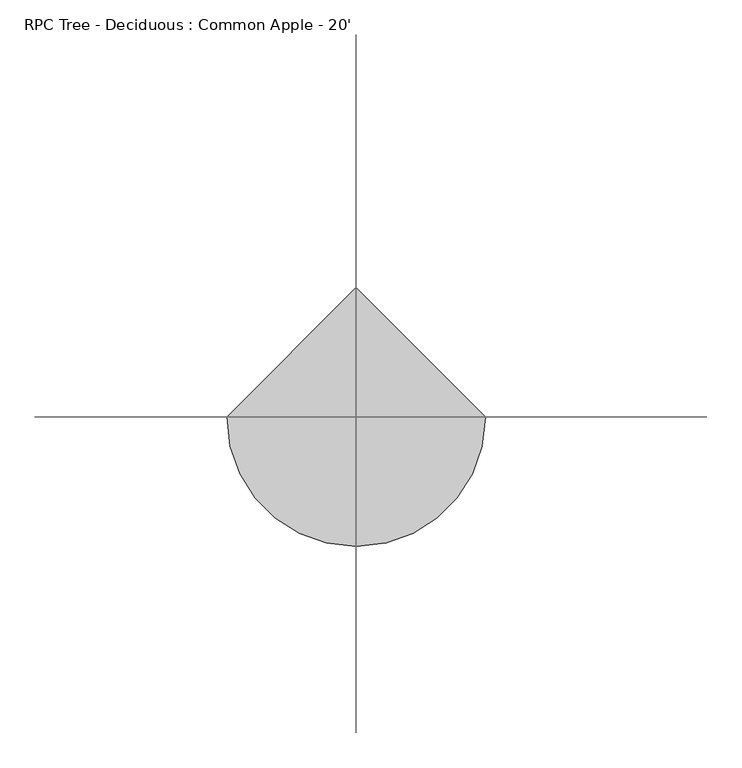
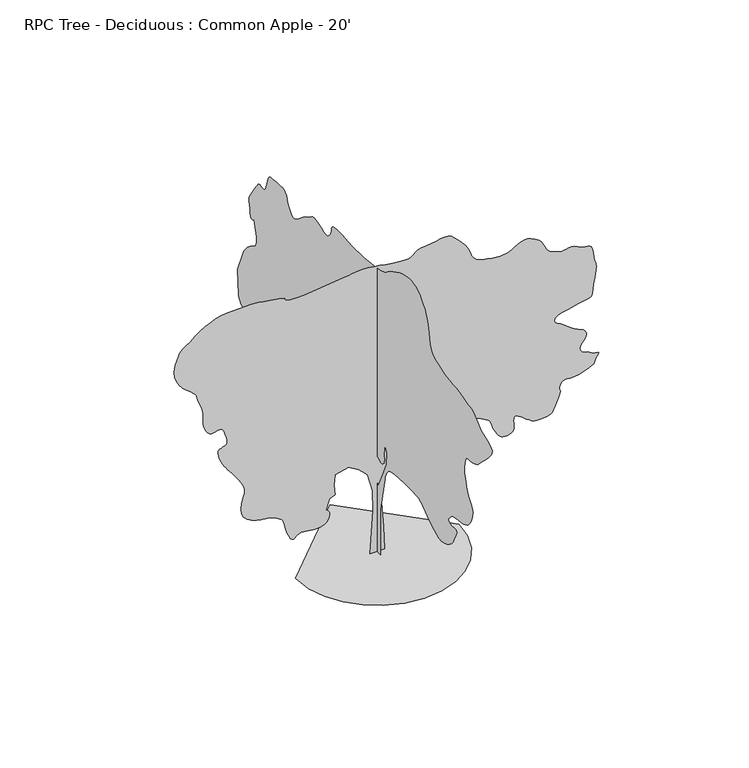
"""IFC4 building model written with IfcOpenShell, lengths in millimetres: geographic element geometry, RPC Tree - Deciduous : Common Apple - 20'."""

from ifc_helpers import new_model, si_unit, origin, place, context, project, spatial, triangles, source, transform, mapped, element, save


def rpc_tree_deciduous_common_apple_20_2cf08d23(model_context):
    return source(origin(), model_context, "Body", "Tessellation", [
        triangles([(-6.61e-05, -106.7031981, 0.0075972), (-6.25e-05, 141.1357166, 0.0075898), (-4.92e-05, 101.4814601, 465.9455781), (-3.19e-05, 131.2220957, 1031.0173004), (-1.83e-05, 230.3576144, 1437.4734501), (-8.7e-06, 398.8869896, 1675.3980263), (-1.1e-06, 587.2459139, 1834.016106), (2.7e-06, 765.6887283, 1873.6680462), (3.6e-06, 963.961219, 1804.2751888), (1.5e-06, 1023.4430534, 1705.1389435), (-4.1e-06, 904.4794573, 1576.2617809), (-8.5e-06, 944.1340136, 1407.7326782), (-1.46e-05, 1172.144878, 1090.4990622), (-1.49e-05, 1568.687534, 882.3128597), (-8.7e-06, 2143.6727863, 803.006436), (7.7e-06, 2490.6473923, 1179.7191977), (2.57e-05, 2847.5453751, 1606.0026981), (3.25e-05, 3402.6882339, 1556.4345028), (3.9e-05, 3600.9610153, 1675.3980263), (4.6e-05, 3591.0549339, 1913.3226025), (4.57e-05, 3412.6196045, 1992.6315697), (5.03e-05, 3283.7399712, 2210.7288677), (5.51e-05, 3591.0549339, 2220.6425068), (6.07e-05, 4205.6845688, 2101.6814541), (6.29e-05, 4275.3567696, 2137.8384041), (6.49e-05, 4342.3114037, 2174.2544952), (6.7e-05, 4403.9061905, 2211.1911942), (6.89e-05, 4457.4241447, 2248.9101128), (7.07e-05, 4500.1976967, 2287.6680668), (7.23e-05, 4529.5348595, 2327.7263775), (7.37e-05, 4542.7427742, 2369.3469475), (8.93e-05, 4572.4863075, 2874.9268433), (9.94e-05, 4403.9570595, 3301.215358), (0.0001002, 4386.5834106, 3334.8449913), (0.000101, 4360.9041641, 3374.6975006), (0.0001018, 4328.265168, 3418.5378479), (0.0001026, 4290.0887192, 3464.105706), (0.0001033, 4247.7471176, 3509.1651649), (0.0001039, 4202.636499, 3551.4561882), (0.0001043, 4156.1291634, 3588.718158), (0.0001045, 4111.323468, 3617.9027138), (0.0001046, 4070.8611122, 3640.1530998), (0.0001046, 4035.4281006, 3659.4571541), (0.0001048, 4005.7101471, 3679.8024239), (0.0001052, 3982.4182549, 3705.2026176), (0.000106, 3966.2384285, 3739.5941231), (0.0001073, 3957.8566727, 3786.9906487), (0.0001089, 3956.7898773, 3842.7945099), (0.0001107, 3961.4378494, 3899.6395866), (0.0001126, 3970.8614021, 3957.3738533), (0.0001145, 3984.0948967, 4015.7685448), (0.0001165, 4000.1982742, 4074.6966339), (0.0001185, 4018.2070587, 4133.9802246), (0.0001206, 4037.1553207, 4193.4417114), (0.0001203, 4062.5299347, 4172.9947037), (0.0001202, 4087.2188347, 4157.4244331), (0.0001204, 4110.5107269, 4151.5570587), (0.000121, 4131.7196068, 4160.2693176), (0.0001221, 4150.160051, 4188.3870781), (0.0001239, 4165.1460548, 4240.787368), (0.0001265, 4175.9410355, 4322.3213448), (0.000129, 4186.6092796, 4402.5600517), (0.0001308, 4198.1408432, 4455.5698975), (0.000132, 4205.3543564, 4492.9588943), (0.000133, 4202.9922913, 4526.3597626), (0.0001339, 4185.923275, 4567.406385), (0.0001352, 4148.8900703, 4627.7059021), (0.000137, 4086.736306, 4718.8666168), (0.0001389, 4019.8834099, 4816.9867905), (0.0001404, 3969.4896835, 4892.043837), (0.0001414, 3931.4405525, 4946.4759796), (0.0001421, 3901.5194138, 4982.6714447), (0.0001423, 3875.5858223, 5003.1184525), (0.0001421, 3849.5002052, 5010.2046478), (0.0001416, 3819.0709579, 5006.343837), (0.0001408, 3787.3208611, 4996.7176804), (0.0001401, 3759.4062859, 4987.6240494), (0.0001396, 3734.2601463, 4983.2045517), (0.0001394, 3710.841227, 4987.6240494), (0.0001396, 3688.1338921, 5005.0485672), (0.0001402, 3665.0704742, 5039.6435486), (0.0001416, 3640.6103394, 5095.574437), (0.0001432, 3619.2235634, 5160.9030075), (0.0001447, 3603.043737, 5219.9581238), (0.000146, 3587.5496246, 5271.4183548), (0.000147, 3568.2455704, 5313.8366959), (0.0001475, 3540.6103386, 5345.8661362), (0.0001475, 3500.1482735, 5366.109668), (0.0001469, 3442.3378487, 5373.1458664), (0.0001459, 3372.4368828, 5376.2445145), (0.0001451, 3300.6055115, 5383.3312912), (0.0001442, 3229.8412262, 5391.1034912), (0.0001434, 3163.0391991, 5396.2851517), (0.0001425, 3103.1713417, 5395.5485687), (0.0001414, 3053.2095657, 5385.642778), (0.0001402, 3016.0746231, 5363.2394943), (0.0001391, 2991.8429626, 5337.2044556), (0.0001382, 2976.4758774, 5316.3510773), (0.0001375, 2966.6462448, 5297.4283951), (0.0001368, 2959.0769394, 5277.1081238), (0.0001359, 2950.4664185, 5252.1148819), (0.0001348, 2937.5122673, 5219.1198029), (0.0001331, 2916.9382324, 5174.873085), (0.0001313, 2890.1666107, 5126.1051315), (0.0001296, 2860.6265533, 5083.2042618), (0.000128, 2827.9619774, 5048.4569641), (0.0001268, 2791.8432518, 5024.124147), (0.0001258, 2751.8890045, 5012.4399765), (0.0001253, 2707.794603, 5015.6909409), (0.0001252, 2659.1789658, 5036.0873703), (0.0001254, 2610.791803, 5068.0662323), (0.0001258, 2565.8846603, 5103.6768494), (0.0001263, 2521.8332794, 5141.7006912), (0.0001267, 2476.0523529, 5180.9436447), (0.0001272, 2425.9356445, 5220.212178), (0.0001274, 2368.8821503, 5258.2360199), (0.0001275, 2302.2908661, 5293.846637), (0.0001276, 2240.2945049, 5328.4671982), (0.0001279, 2193.5584042, 5362.0459625), (0.0001282, 2154.2798424, 5391.129071), (0.0001282, 2114.6558075, 5412.2365036), (0.0001278, 2066.8783459, 5421.8882401), (0.0001267, 2003.1496777, 5416.6304214), (0.0001247, 1915.6618492, 5392.9830276), (0.0001224, 1826.1497257, 5361.2837997), (0.0001207, 1757.9710384, 5335.9853439), (0.0001194, 1705.7434124, 5319.8816757), (0.0001187, 1664.0950825, 5315.7418121), (0.0001184, 1627.6484699, 5326.358606), (0.0001187, 1591.0293388, 5354.4766571), (0.0001195, 1548.8602558, 5402.8893997), (0.0001207, 1514.8419834, 5459.7853455), (0.000122, 1498.8602554, 5510.7630478), (0.0001232, 1489.8128426, 5554.806871), (0.0001241, 1476.6047825, 5590.874437), (0.0001244, 1448.1338459, 5617.9256927), (0.0001241, 1393.3079773, 5634.9182602), (0.0001229, 1301.0220406, 5640.8109238), (0.0001214, 1201.3955635, 5639.6935501), (0.0001202, 1126.7398006, 5636.6454803), (0.0001192, 1069.2519579, 5632.2259827), (0.0001184, 1021.1290958, 5626.9425842), (0.0001175, 974.5682751, 5621.3039749), (0.0001165, 921.7642307, 5615.8426804), (0.0001154, 854.9113346, 5611.0679718), (0.0001143, 784.7082069, 5608.019902), (0.0001133, 723.0014357, 5607.2071609), (0.0001125, 663.7228592, 5608.4768509), (0.0001116, 600.8019178, 5611.6516571), (0.0001107, 528.1680156, 5616.5792633), (0.0001096, 439.7556433, 5623.0567749), (0.0001082, 329.4941322, 5630.9051331), (0.0001067, 206.9466705, 5641.7254028), (0.0001053, 88.3885184, 5656.6861176), (0.0001042, -22.1921751, 5675.1262711), (0.0001034, -120.8075788, 5696.3354416), (0.0001029, -203.4686488, 5719.6276245), (0.0001027, -266.1871316, 5744.3162338), (0.0001028, -304.9729546, 5769.6908478), (0.0001032, -347.9523442, 5804.4381454), (0.0001036, -420.583703, 5853.4089935), (0.0001039, -514.8939712, 5910.1532043), (0.000104, -622.9024584, 5968.31884), (0.0001039, -736.6335978, 6021.4301331), (0.0001035, -848.1092062, 6063.1118912), (0.0001027, -949.3562239, 6086.9371811), (0.0001016, -1039.2697763, 6095.8017563), (0.0001004, -1122.4243664, 6096.0046509), (9.9e-05, -1199.3330441, 6086.1494385), (9.73e-05, -1270.5191059, 6064.8391113), (9.53e-05, -1336.5033051, 6030.7016602), (9.29e-05, -1397.8062492, 5982.3650757), (9.01e-05, -1454.9462208, 5918.407933), (8.77e-05, -1502.3755932, 5861.1056168), (8.62e-05, -1536.9730453, 5825.4944183), (8.5e-05, -1562.8963177, 5799.256485), (8.38e-05, -1584.313615, 5770.0716385), (8.22e-05, -1605.3828232, 5725.6220261), (7.96e-05, -1630.2698215, 5653.5874695), (7.58e-05, -1663.1323505, 5541.6751144), (7.16e-05, -1693.8258259, 5415.6147858), (6.81e-05, -1715.6747829, 5307.5626602), (6.5e-05, -1738.0446384, 5214.9799393), (6.21e-05, -1770.3000824, 5135.1981812), (5.93e-05, -1821.8062408, 5065.6530075), (5.62e-05, -1901.9230076, 5003.7532974), (5.28e-05, -2020.0178341, 4946.8823502), (4.95e-05, -2152.913356, 4902.7117905), (4.69e-05, -2273.494804, 4876.3974083), (4.48e-05, -2385.2295536, 4861.5384315), (4.29e-05, -2491.5921021, 4851.7340881), (4.1e-05, -2596.0345642, 4840.5071571), (3.89e-05, -2702.0542557, 4821.482737), (3.62e-05, -2813.1030006, 4788.2594742), (3.39e-05, -2912.3155495, 4758.5159409), (3.24e-05, -2986.585144, 4746.9843773), (3.14e-05, -3044.8780975, 4742.742485), (3.04e-05, -3096.2371719, 4734.8432579), (2.89e-05, -3149.6786774, 4712.3896866), (2.66e-05, -3214.2200867, 4664.4344742), (2.28e-05, -3298.878582, 4580.0809021), (1.85e-05, -3408.6320572, 4492.8062874), (1.5e-05, -3530.0185432, 4434.3354378), (1.2e-05, -3644.3188339, 4390.95233), (9.4e-06, -3732.7616913, 4348.9659393), (7.2e-06, -3776.6273277, 4294.6608238), (5.1e-06, -3757.196537, 4214.3459587), (3e-06, -3655.7486595, 4094.3056114), (1.1e-06, -3529.027906, 3968.7786804), (-3e-07, -3439.3912262, 3876.7287758), (-1.3e-06, -3376.6531952, 3811.5525215), (-1.9e-06, -3330.5522301, 3766.670668), (-2.3e-06, -3290.852037, 3735.479258), (-2.3e-06, -3247.3671913, 3711.4002045), (-2.2e-06, -3189.8108208, 3687.854258), (-1.7e-06, -3124.3802216, 3671.1919029), (-1e-06, -3064.487075, 3666.3404549), (-2e-07, -3010.8420937, 3664.4356293), (2e-07, -2964.1568619, 3656.6378494), (2e-07, -2925.0662247, 3634.0825401), (-8e-07, -2894.3070557, 3587.9559952), (-2.8e-06, -2872.5897766, 3509.3939301), (-5.1e-06, -2860.8041588, 3423.8465355), (-7.1e-06, -2858.3659355, 3357.9081184), (-8.8e-06, -2863.7507813, 3304.4410332), (-1.04e-05, -2875.358503, 3256.3335045), (-1.21e-05, -2891.6653564, 3206.498465), (-1.41e-05, -2911.070858, 3147.8244301), (-1.67e-05, -2932.0768433, 3073.199334), (-1.95e-05, -2961.2613991, 2993.8242371), (-2.22e-05, -3001.7234642, 2923.6186386), (-2.47e-05, -3046.5291595, 2859.6612053), (-2.72e-05, -3088.7187355, 2798.9806068), (-2.95e-05, -3121.3830208, 2738.6555099), (-3.16e-05, -3137.5628471, 2675.7398735), (-3.35e-05, -3130.349334, 2607.2612045), (-3.52e-05, -3109.3942177, 2540.281572), (-3.66e-05, -3087.7280983, 2482.819091), (-3.77e-05, -3063.4964378, 2433.5098915), (-3.85e-05, -3034.7182526, 2390.964814), (-3.91e-05, -2999.5645844, 2353.7970245), (-3.94e-05, -2956.0544495, 2320.6169277), (-3.96e-05, -2902.3333099, 2290.0378349), (-3.93e-05, -2836.3948929, 2266.2507694), (-3.86e-05, -2760.9314758, 2251.4832115), (-3.77e-05, -2680.9721123, 2241.3942924), (-3.68e-05, -2601.4955681, 2231.6559334), (-3.61e-05, -2527.6041481, 2217.9272655), (-3.58e-05, -2464.279525, 2195.8749779), (-3.62e-05, -2416.56049, 2161.1632885), (-3.68e-05, -2383.2356346, 2123.2410393), (-3.73e-05, -2359.9691769, 2093.2995529), (-3.79e-05, -2347.1065899, 2069.598674), (-3.84e-05, -2344.9984337, 2050.4090023), (-3.9e-05, -2353.9875652, 2033.9929985), (-3.98e-05, -2374.4217831, 2018.6158848), (-4.07e-05, -2406.646851, 2002.5452087), (-4.16e-05, -2449.8269188, 1993.9041664), (-4.23e-05, -2498.3841293, 1996.5330757), (-4.28e-05, -2545.5646797, 2002.2862129), (-4.34e-05, -2584.5791588, 2003.0075352), (-4.41e-05, -2608.6837921, 1990.5513187), (-4.52e-05, -2611.0967262, 1956.7642822), (-4.66e-05, -2585.0869766, 1893.4953243), (-4.83e-05, -2549.9080193, 1821.1814243), (-4.96e-05, -2524.6272949, 1762.91376), (-5.07e-05, -2502.1126808, 1714.5318295), (-5.16e-05, -2475.2625755, 1671.8725147), (-5.23e-05, -2436.9668026, 1630.7726978), (-5.27e-05, -2380.1140228, 1587.0720222), (-5.3e-05, -2297.5969666, 1536.6072247), (-5.28e-05, -2203.8378639, 1496.8968578), (-5.19e-05, -2116.842738, 1484.7582092), (-5.03e-05, -2034.8743401, 1494.9892708), (-4.83e-05, -1956.2028339, 1522.3883251), (-4.6e-05, -1879.090971, 1561.7532188), (-4.35e-05, -1801.803828, 1607.8822346), (-4.09e-05, -1722.6115688, 1655.5707481), (-3.83e-05, -1647.9584221, 1703.6352562), (-3.59e-05, -1583.013113, 1752.3931812), (-3.37e-05, -1524.1383636, 1798.8980461), (-3.16e-05, -1467.6919544, 1840.2010483), (-2.97e-05, -1410.0313751, 1873.3506237), (-2.82e-05, -1347.5167316, 1895.4053822), (-2.69e-05, -1276.503479, 1903.4089634), (-2.54e-05, -1177.6846561, 1904.2776604), (-2.33e-05, -1044.3574018, 1905.4916851), (-2.11e-05, -891.7820492, 1904.9710773), (-1.89e-05, -735.2163151, 1900.6352955), (-1.7e-05, -589.9230761, 1890.4040886), (-1.58e-05, -471.1627742, 1872.1948803), (-1.55e-05, -394.1956335, 1843.9297451), (-1.6e-05, -348.7041879, 1805.3140789), (-1.68e-05, -313.0958962, 1758.377409), (-1.8e-05, -285.7248199, 1704.5039532), (-1.95e-05, -264.9450744, 1645.0805454), (-2.11e-05, -249.1058704, 1581.494165), (-2.29e-05, -236.5620685, 1515.1341167), (-2.48e-05, -225.6659676, 1447.3870892), (-3.91e-05, -116.6168281, 912.0537769), (-2.05e-05, -27.3946828, 1318.5099266), (-1.32e-05, -176.0980811, 1635.74347), (-6.6e-06, -304.975498, 1923.2362415), (2e-07, -324.8002327, 2161.1632885), (4.8e-06, -255.4073572, 2280.1241959), (-4e-07, -225.6657133, 2091.767815), (-1.7e-06, -231.7353101, 2049.4539734), (-3e-06, -235.984215, 2008.1814926), (-4.2e-06, -236.5910275, 1968.9892628), (-5.2e-06, -231.7353101, 1932.9186447), (-6e-06, -219.5961346, 1901.0111446), (-6.5e-06, -198.3530817, 1874.3056526), (-6.6e-06, -166.1844602, 1853.8433842), (-6.2e-06, -129.2182845, 1848.5829494), (-5.3e-06, -95.0268123, 1860.3152275), (-4.3e-06, -63.9562343, 1879.3348515), (-3.4e-06, -36.354542, 1895.9235191), (-2.9e-06, -12.5678035, 1900.3761543), (-3.1e-06, 7.0569383, 1882.9772163), (-4.4e-06, 22.1729471, 1834.016106), (-6.1e-06, 32.8958209, 1768.9260384), (-7.8e-06, 39.9768386, 1709.0403042), (-9.4e-06, 44.0233167, 1653.4904972), (-1.1e-05, 45.6418044, 1601.4077751), (-1.24e-05, 45.4396183, 1551.9260571), (-1.39e-05, 44.0233167, 1504.1789715), (-1.53e-05, 41.9999482, 1457.3007282), (139.590126, 0.0003305, 0.0), (-135.4471285, 0.0003387, 0.0), (-74.3278259, 0.000241, 845.4879272), (-84.5142454, 0.0002472, 1242.76455), (-186.3807747, 0.0002013, 1599.294532), (-339.1791879, 0.0002082, 1752.0933449), (-542.9102117, 0.000216, 1874.3335579), (-797.5758808, 0.0002227, 1813.2134514), (-817.9492012, 0.0002203, 1609.4824276), (-797.5758808, 0.0002168, 1415.9368286), (-899.4426281, 0.0002191, 1365.0021469), (-970.7481594, 0.0002183, 1171.4565479), (-951.3247084, 0.0002718, 1158.1240768), (-933.2373676, 0.000271, 1143.3616058), (-917.8246456, 0.0002703, 1125.7517796), (-906.4200365, 0.0002696, 1103.8645981), (-900.3621214, 0.000269, 1076.2750757), (-900.9870106, 0.0002686, 1041.555756), (-909.6280529, 0.0002682, 998.2868128), (-928.5764603, 0.0002681, 955.1042742), (-957.6798437, 0.0002684, 921.0098436), (-994.6267164, 0.0002692, 895.1144766), (-1037.0955631, 0.0002701, 876.5217161), (-1082.7698101, 0.0002713, 864.3449158), (-1129.3382612, 0.0002726, 857.6926329), (-1174.4791832, 0.0002739, 855.6733521), (-1218.6700905, 0.0002753, 858.4063974), (-1263.5747623, 0.0002767, 865.0586803), (-1308.6573303, 0.0002782, 873.3161705), (-1353.3816353, 0.0002796, 880.857498), (-1397.217041, 0.000281, 885.3710306), (-1439.6273884, 0.0002823, 884.5404854), (-1480.0769543, 0.0002833, 876.0466724), (-1514.854628, 0.0002841, 857.900905), (-1542.5051205, 0.0002846, 834.4084436), (-1565.8782578, 0.000285, 812.6990856), (-1587.8238659, 0.0002854, 799.9000122), (-1611.1970032, 0.0002862, 803.1359339), (-1638.8473503, 0.0002874, 829.5392641), (-1673.6225533, 0.000235, 886.2346407), (-1706.6171963, 0.0002371, 959.4984827), (-1729.2790398, 0.0002388, 1029.5593225), (-1744.988982, 0.0002402, 1094.4487484), (-1757.1353336, 0.0002415, 1152.2135365), (-1769.1037891, 0.0002426, 1200.8900711), (-1784.2803337, 0.0002436, 1238.5177162), (-1806.0481911, 0.0002446, 1263.1378704), (-1833.1626698, 0.0002457, 1282.7670502), (-1863.3073414, 0.0002469, 1305.4288937), (-1898.2629112, 0.0002483, 1329.1576778), (-1939.8122646, 0.0002499, 1351.9948013), (-1989.7334908, 0.0002517, 1371.9820988), (-2049.8147072, 0.0002537, 1387.1586433), (-2121.8338577, 0.000256, 1395.5635082), (-2205.4938675, 0.0002044, 1404.6210949), (-2294.67854, 0.0002073, 1424.3695988), (-2382.4381542, 0.0002104, 1456.7724174), (-2461.8232796, 0.0002135, 1503.7853909), (-2525.8821602, 0.0002163, 1567.3691551), (-2567.6627495, 0.0002188, 1649.4849277), (-2580.2355286, 0.0002207, 1752.0933449), (-2568.9835991, 0.0002218, 1851.4048702), (-2548.8159348, 0.0002224, 1927.9097935), (-2527.0379036, 0.0002227, 1989.979842), (-2510.9723145, 0.0001688, 2045.9893593), (-2507.9117455, 0.0001695, 2104.3180664), (-2525.1659248, 0.0001711, 2173.3375454), (-2570.0503944, 0.0001737, 2261.4222851), (-2629.7912247, 0.0001769, 2355.7756828), (-2686.3316689, 0.0001798, 2438.7243988), (-2738.9604332, 0.0001825, 2511.3356644), (-2786.9665146, 0.0001849, 2574.6730774), (-2829.6130394, 0.0001327, 2629.841803), (-2866.1890045, 0.0001345, 2677.8478844), (-2896.008696, 0.000136, 2719.8086952), (-2924.6092758, 0.0001376, 2767.4084061), (-2955.1652596, 0.0001394, 2827.2762634), (-2983.4100471, 0.0001412, 2893.0114952), (-3005.0764572, 0.0001428, 2958.2389091), (-3015.8461487, 0.000144, 3016.5062828), (-3011.4772293, 0.0001446, 3061.4137161), (-2987.7028084, 0.0001442, 3086.5342758), (-2951.4823448, 0.0001433, 3098.8532913), (-2915.109565, 0.0001425, 3111.5533882), (-2882.1147766, 0.0001417, 3127.4282913), (-2856.0800285, 0.0001413, 3149.3740448), (-2840.5350471, 0.0001413, 3180.2349518), (-2839.0871704, 0.0001418, 3222.8561874), (-2855.2669968, 0.0001432, 3280.0823456), (-2877.0348541, 9.05e-05, 3338.9342766), (-2892.2240433, 9.16e-05, 3385.5177704), (-2904.1875572, 9.25e-05, 3421.2048363), (-2916.3286766, 9.32e-05, 3447.4686401), (-2932.0259743, 9.4e-05, 3465.705899), (-2954.70802, 9.48e-05, 3477.3389099), (-2987.7028084, 9.59e-05, 3483.8161308), (-3026.4123642, 9.7e-05, 3481.8857254), (-3064.2583099, 9.8e-05, 3472.1066711), (-3101.5455688, 9.9e-05, 3461.6419029), (-3138.6805115, 0.0001, 3457.552327), (-3175.9930595, 0.0001013, 3467.026458), (-3213.8137161, 0.0001029, 3497.1763618), (-3252.5488518, 0.0001049, 3555.1138138), (-3281.1747208, 0.0001068, 3626.7419998), (-3293.239682, 0.0001082, 3695.3474052), (-3295.8558014, 0.0001093, 3764.1307068), (-3296.1351448, 0.0001104, 3836.3175797), (-3301.2406471, 5.74e-05, 3915.0575409), (-3318.2840836, 5.93e-05, 4003.6274254), (-3354.4028091, 6.19e-05, 4105.2020393), (-3391.2836975, 6.43e-05, 4197.0231789), (-3411.2481766, 6.59e-05, 4259.8120789), (-3422.2972115, 6.68e-05, 4301.925206), (-3432.4570564, 6.76e-05, 4331.7448975), (-3449.7545471, 6.85e-05, 4357.6276199), (-3482.1650688, 6.99e-05, 4387.9804184), (-3537.7657448, 7.22e-05, 4431.1606316), (-3609.6985634, 2.09e-05, 4488.5646858), (-3681.631382, 2.41e-05, 4556.1285851), (-3747.3157448, 2.72e-05, 4634.0305161), (-3800.5287758, 3.01e-05, 4722.4480843), (-3835.047599, 3.26e-05, 4821.5588951), (-3844.6231773, 3.45e-05, 4931.5152649), (-3822.9823471, 3.57e-05, 5052.5468307), (-3789.555899, -1.8e-05, 5157.9310959), (-3763.7749146, -1.77e-05, 5228.187854), (-3739.5941231, -1.77e-05, 5274.3902664), (-3710.9682541, -1.81e-05, 5307.5882401), (-3671.8270386, -1.88e-05, 5338.8555176), (-3616.1246246, -1.98e-05, 5379.1652664), (-3537.7657448, -2.13e-05, 5439.6429703), (-3445.4364967, -2.3e-05, 5511.6775269), (-3351.6849518, -2.48e-05, 5578.225209), (-3256.3079247, -2.67e-05, 5637.4326416), (-3159.1783882, -2.89e-05, 5687.5726044), (-3060.0675774, -3.12e-05, 5726.8155579), (-2958.8228851, -3.39e-05, 5753.4348633), (-2855.2669968, -3.68e-05, 5765.6015625), (-2376.4970924, -5.09e-05, 5775.7869873), (-2309.7356152, -5.29e-05, 5773.1197083), (-2232.8167637, -5.53e-05, 5765.6521408), (-2147.4320045, -3.8e-06, 5754.1458664), (-2055.2781818, -6.7e-06, 5739.4392059), (-1958.0469074, -9.9e-06, 5722.3449005), (-1857.4273224, -1.32e-05, 5703.6251129), (-1755.1159801, -1.65e-05, 5684.1181641), (-1751.9080364, -1.69e-05, 5664.6617935), (-1742.5530842, -1.75e-05, 5646.3739563), (-1720.9022255, -1.83e-05, 5630.3970245), (-1680.8107773, -1.97e-05, 5617.9001129), (-1616.1270802, -2.18e-05, 5610.0261749), (-1520.7042709, -2.46e-05, 5607.9437439), (-1388.3981026, -2.85e-05, 5612.8201904), (-614.2181774, -5.02e-05, 5704.4890137), (-538.3076946, -5.24e-05, 5711.4996323), (-472.1990845, 1e-07, 5721.8879517), (-409.4762778, -1.6e-06, 5732.8355392), (-343.7232419, -3.5e-06, 5741.4460602), (-268.5264692, -5.7e-06, 5744.8749207), (-177.4707081, -8.5e-06, 5740.3031067), (-64.1414019, -1.21e-05, 5724.8598633), (54.7118994, -1.59e-05, 5704.3111176), (159.4882483, -1.93e-05, 5686.4296509), (252.3260954, -2.23e-05, 5671.4183578), (335.3640864, -2.49e-05, 5659.4039749), (410.7386644, -2.73e-05, 5650.6155579), (480.5886887, -2.95e-05, 5645.205423), (547.0529457, -3.15e-05, 5643.3764648), (603.2428662, -3.3e-05, 5651.8346695), (646.0698669, -3.4e-05, 5673.6531052), (683.3697704, -3.47e-05, 5703.4983765), (722.9887184, -3.54e-05, 5736.0359253), (772.7625698, -3.64e-05, 5765.8806152), (840.5349592, -3.81e-05, 5787.6996323), (934.1441437, -4.07e-05, 5796.1828354), (1035.6832947, -4.37e-05, 5802.989978), (1124.0372766, -4.61e-05, 5818.3826431), (1202.2337391, -4.82e-05, 5834.6642075), (1273.3004768, -5.01e-05, 5844.1636276), (1340.2726971, -5.22e-05, 5839.2360214), (1406.173035, -5.46e-05, 5812.2103455), (1474.0342999, -3.2e-06, 5755.4161377), (1539.0152172, -6.2e-06, 5686.9627579), (1594.7301304, -8.7e-06, 5628.1366974), (1641.8903332, -1.09e-05, 5576.0666199), (1681.2120609, -1.28e-05, 5527.9335114), (1713.4041367, -1.44e-05, 5480.8671982), (1739.182505, -1.59e-05, 5431.9975067), (1759.2587505, -1.73e-05, 5378.5304214), (1777.3156425, -1.87e-05, 5324.8604416), (1798.9361252, -2e-05, 5277.2604401), (1827.6839344, -2.15e-05, 5235.5281036), (1867.1225155, 3.1e-05, 5199.4855362), (1920.8180752, 2.9e-05, 5169.0060013), (1992.3318787, 2.65e-05, 5143.8342819), (2085.229842, 2.34e-05, 5123.844223), (2181.6306438, 2.03e-05, 5109.4171967), (2262.7075264, 1.78e-05, 5100.6799393), (2330.5991673, 1.57e-05, 5097.123761), (2387.4419186, 1.4e-05, 5098.1905563), (2435.3767834, 1.27e-05, 5103.3722168), (2476.5374977, 1.16e-05, 5112.0844757), (2513.0678261, 1.07e-05, 5123.844223), (2552.2195061, 9.8e-06, 5144.4947067), (2599.1840813, 8.9e-06, 5175.4829315), (2653.1336952, 7.8e-06, 5209.6459625), (2713.1032906, 6.4e-06, 5239.9226028), (2778.2795448, 4.8e-06, 5259.1249191), (2847.697982, 2.7e-06, 5260.1661346), (2920.5196999, 2e-07, 5235.9094757), (2984.2992371, -2.2e-06, 5202.1528152), (3030.2478859, -4e-06, 5176.5747253), (3062.9883293, -5.3e-06, 5154.908606), (3087.1947006, -6.3e-06, 5132.9122742), (3107.4893921, -7.3e-06, 5106.2679703), (3128.4697975, -8.5e-06, 5070.73293), (3154.8094688, -1e-05, 5021.9905563), (3182.8510712, 4.27e-05, 4971.0890121), (3208.2256851, 4.13e-05, 4930.3473129), (3234.4639091, 4e-05, 4897.4289734), (3265.1724998, 3.87e-05, 4870.0475052), (3303.9076355, 3.72e-05, 4845.8667137), (3354.2252037, 3.53e-05, 4822.6004013), (3419.6808014, 3.3e-05, 4797.8859215), (3486.0258797, 3.08e-05, 4782.8237595), (3540.0769409, 2.92e-05, 4784.7032959), (3586.9909378, 2.8e-05, 4795.4729874), (3631.9489494, 2.68e-05, 4807.1571579), (3680.1326363, 2.55e-05, 4811.7036827), (3736.6730804, 2.36e-05, 4801.0863075), (3806.7519424, 2.1e-05, 4767.3299377), (3879.2181587, 1.84e-05, 4732.9890106), (3939.9240463, 1.63e-05, 4718.4346664), (3989.5811897, 1.48e-05, 4712.2626595), (4028.9003014, 1.35e-05, 4703.0678719), (4058.6185455, 1.22e-05, 4679.4204781), (4079.3957657, 6.51e-05, 4629.9412308), (4091.9941246, 6.34e-05, 4543.2253029), (4103.8306114, 6.18e-05, 4454.6301292), (4119.4261711, 6.04e-05, 4397.0481789), (4135.0217308, 5.94e-05, 4355.3161331), (4146.8835068, 5.84e-05, 4314.2950905), (4151.2268463, 5.74e-05, 4258.8467308), (4144.3688347, 5.64e-05, 4173.8330246), (4122.550399, 5.51e-05, 4044.0642014), (4100.096537, 0.000108, 3908.7329269), (4088.8698967, 0.0001069, 3812.0603394), (4081.3767494, 0.0001061, 3746.5791618), (4070.1501091, 0.0001058, 3704.7962471), (4047.6965378, 0.0001061, 3679.2184479), (4006.548468, 0.0001071, 3662.4034859), (3939.1874634, 0.0001089, 3646.8079262), (3844.4708611, 0.0001114, 3628.5706673), (3734.0822502, 0.0001144, 3608.1998177), (3619.7822502, 0.0001175, 3584.781189), (3513.3053192, 0.0001202, 3557.4761696), (3426.4373657, 0.0001224, 3525.3449913), (3370.9384277, 0.0001234, 3487.4990456), (3358.5429634, 0.0001231, 3443.0744316), (3371.5224037, 0.0001222, 3405.6092766), (3386.2799332, 0.0001214, 3384.1972115), (3405.8633308, 0.0001207, 3371.1669022), (3433.2700882, 0.0001197, 3358.8478867), (3471.5476936, 0.0001182, 3339.5694122), (3523.7447983, 0.0001162, 3305.6857246), (3592.8327324, 0.0001133, 3249.5260712), (3669.2870773, 0.0001101, 3189.9884262), (3740.381575, 0.0001074, 3147.3671906), (3804.5419029, 0.000105, 3116.150782), (3860.1425789, 0.0001572, 3090.8014572), (3905.55783, 0.0001555, 3065.8332138), (3939.2383324, 0.000154, 3035.6833099), (3959.558313, 0.0001528, 2994.8654526), (3960.2948959, 0.0001521, 2946.884951), (3941.8038734, 0.0001519, 2899.2852402), (3912.2635254, 0.0001521, 2852.3968231), (3879.8530037, 0.0001524, 2806.5752014), (3852.8020386, 0.0001525, 2762.1758766), (3839.2892006, 0.0001523, 2719.554641), (3847.5189308, 0.0001514, 2679.0672867), (3870.582058, 0.0001503, 2647.1645828), (3896.1598572, 0.0001492, 2627.2256836), (3924.2270393, 0.0001482, 2614.9319572), (3954.7830231, 0.0001472, 2606.0168037), (3987.8286804, 0.000146, 2596.2121696), (4023.3887192, 0.0001447, 2581.2517456), (4061.4378502, 0.0001432, 2556.842189), (4100.7569618, 0.0001417, 2534.5891869), (4137.7648773, 0.0001405, 2524.8203064), (4168.8798386, 0.0001395, 2521.2847664), (4190.5462486, 0.0001388, 2517.7515518), (4199.2329277, 0.0001384, 2507.9803459), (4191.3334099, 0.0001926, 2485.7375175), (4163.2918076, 0.0001928, 2444.7824593), (4135.3263634, 0.0001929, 2399.7888393), (4122.8550316, 0.0001928, 2366.7332989), (4115.1842789, 0.0001927, 2341.3408081), (4101.6461517, 0.0001927, 2319.3343025), (4071.521537, 0.0001933, 2296.4387524), (4014.1430626, 0.0001946, 2268.3717155), (3918.8166138, 0.0001969, 2230.8633945), (3811.1205711, 0.0001996, 2200.6297749), (3722.1443161, 0.0002021, 2191.0666958), (3649.3987564, 0.0002043, 2192.9081532), (3590.3436401, 0.0002062, 2196.8884335), (3542.540744, 0.0002075, 2193.7413872), (3503.4501068, 0.0002084, 2174.1985394), (3470.6079254, 0.0002087, 2128.9966473), (3451.2532928, 0.0002086, 2081.7474964), (3449.1702805, 0.0002083, 2055.3443115), (3456.7142967, 0.0002078, 2039.4564732), (3466.2137169, 0.0002073, 2023.7466763), (3470.0236588, 0.0002068, 1997.8792145), (3460.4480804, 0.0002064, 1951.5191082), (3429.8662262, 0.0002061, 1874.3335579), (3393.2393921, 0.0002059, 1787.376511), (3366.4171921, 0.0002057, 1717.5239433), (3342.9982727, 0.0002056, 1663.1755165), (3316.5315742, 0.0002058, 1622.7259506), (3280.6157433, 0.0002064, 1594.5725819), (3228.850589, 0.0002077, 1577.1101303), (3154.8094688, 0.0002098, 1568.7357868), (3080.6413216, 0.0002119, 1565.2609989), (3027.8349518, 0.0002135, 1564.6361824), (2989.0998161, 0.0002147, 1568.469088), (2957.146534, 0.0002158, 1578.3572926), (2924.6598541, 0.000217, 1595.9086922), (2884.3248161, 0.0002186, 1622.7259506), (2828.8511673, 0.0002209, 1660.4146385), (2768.830703, 0.0002233, 1702.4363468), (2719.1482704, 0.0002253, 1739.6499184), (2678.9146797, 0.000227, 1769.7336926), (2647.2154518, 0.0002282, 1790.3763279), (2623.1869766, 0.0002291, 1799.2561638), (2605.9403549, 0.0002295, 1794.0567719), (2594.5613983, 0.0002295, 1772.4668106), (2588.1350464, 0.0002293, 1744.7273701), (2585.6459541, 0.000229, 1721.445797), (2586.0014557, 0.0002287, 1700.833683), (2588.1350464, 0.0002283, 1681.1130844), (2591.00522, 0.0002279, 1660.5034412), (2593.494603, 0.0002275, 1637.219252), (2594.5613983, 0.0002271, 1609.4824276), (2593.1135216, 0.0002267, 1579.0989624), (2587.906572, 0.0002264, 1549.7873795), (2577.7211472, 0.0002263, 1522.6143288), (2561.2872665, 0.0002264, 1498.6468964), (2537.3884346, 0.0002268, 1478.9568192), (2504.7494385, 0.0002276, 1464.6108925), (2462.1331444, 0.0002288, 1456.6836147), (2418.7144283, 0.00023, 1454.9893867), (2382.9562912, 0.0002312, 1459.35569), (2352.5447754, 0.0002322, 1470.8491745), (2325.1635979, 0.0002333, 1490.5392517), (2298.4935688, 0.0002346, 1519.4951878), (2270.2207306, 0.000236, 1558.7865395), (2238.0288002, 0.0002377, 1609.4824276), (2208.2396301, 0.0002394, 1664.8392231), (2186.8274197, 0.0001866, 1716.8127949), (2170.9397266, 0.0001878, 1764.5088661), (2157.7241089, 0.0001888, 1807.0362122), (2144.3307404, 0.0001897, 1843.5054977), (2127.9070335, 0.0001907, 1873.0254982), (2105.6033077, 0.0001917, 1894.7068783), (2074.6583942, 0.0001929, 1913.6528149), (2035.1589157, 0.0001944, 1935.2732975), (1988.5319653, 0.0001961, 1959.1214058), (1936.2028919, 0.0001981, 1984.7525448), (1879.5964634, 0.0002001, 2011.717178), (1820.1400635, 0.0002023, 2039.5759426), (1759.2587505, 0.0002046, 2067.8791569), (1412.9141933, 0.0002149, 2067.8791569), (1219.3685944, 0.0002173, 1843.7721966), (1214.8270838, 0.000217, 1813.2134514), (1209.2136909, 0.0002167, 1782.6522354), (1201.4616205, 0.0002165, 1752.0933449), (1190.5040045, 0.0002164, 1721.5345997), (1175.2665625, 0.0002164, 1690.9733837), (1154.6874407, 0.0002165, 1660.4146385), (1127.6898153, 0.0002169, 1629.855748), (1103.6638836, 0.0002172, 1604.0163368), (1088.903956, 0.0002174, 1586.5538853), (1077.7076191, 0.0002175, 1575.8629681), (1064.3726046, 0.0002179, 1570.3384506), (1043.1966442, 0.0002185, 1568.3775238), (1008.4798679, 0.0002195, 1568.3775238), (954.5175367, 0.0002211, 1568.7357868), (886.9839409, 0.0002232, 1571.6161343), (817.1339167, 0.0002254, 1579.3072346), (747.6394667, 0.0002276, 1590.3841747), (681.1726662, 0.0002298, 1603.4220417), (620.41075, 0.0002318, 1616.9957771), (568.0206702, 0.0002335, 1629.6755264), (526.6821324, 0.0002349, 1640.0411728), (491.1627162, 0.0002361, 1650.5543392), (454.5739975, 0.0002374, 1664.275304), (417.0937271, 0.0002388, 1680.6684895), (378.9022719, 0.0002402, 1699.2003525), (340.1748393, 0.0001874, 1719.3350246), (301.0918324, 0.0001889, 1740.5414337), (261.828495, 0.0001904, 1762.2813858), (78.4708189, 0.0002443, 1375.1901878), (68.2843994, 0.0002402, 1079.7776962), (119.217278, 0.0002837, 458.3966929), (-1547.0796959, 1.1e-06, 0.0099807), (-1506.1805935, -354.4877738, 0.0099913), (-1389.6986046, -680.02964, 0.010001), (-1206.9607035, -967.2962626, 0.0100095), (-967.2962626, -1206.9607035, 0.0100167), (-680.02964, -1389.6986046, 0.0100221), (-354.4877738, -1506.1805935, 0.0100256), (6.76e-05, -1547.0796959, 0.0100268), (354.4877738, -1506.1805935, 0.0100256), (680.02964, -1389.6986046, 0.0100221), (967.2962626, -1206.9607035, 0.0100167), (1206.9607035, -967.2962626, 0.0100095), (1389.6986046, -680.02964, 0.010001), (1506.1805935, -354.4877738, 0.0099913), (1547.0796959, 0.0001258, 0.0099807), (-0.0002029, 1547.0796959, 0.0099346)], [[300, 1, 301], [299, 300, 301], [299, 301, 302], [298, 299, 302], [297, 298, 302], [296, 297, 302], [296, 302, 303], [295, 296, 303], [294, 295, 303], [293, 294, 303], [292, 293, 303], [1, 2, 3], [301, 1, 3], [301, 3, 4], [301, 4, 5], [327, 301, 5], [326, 327, 5], [326, 5, 6], [325, 326, 6], [324, 325, 6], [323, 324, 6], [322, 323, 6], [321, 322, 6], [320, 321, 6], [19, 20, 21], [18, 19, 21], [17, 18, 21], [17, 21, 22], [320, 6, 7], [319, 320, 7], [291, 292, 303], [291, 303, 304], [290, 291, 304], [261, 262, 263], [260, 261, 263], [260, 263, 264], [259, 260, 264], [259, 264, 265], [258, 259, 265], [10, 11, 12], [14, 15, 16], [258, 265, 266], [257, 258, 266], [205, 206, 207], [204, 205, 207], [204, 207, 208], [203, 204, 208], [203, 208, 209], [202, 203, 209], [202, 209, 210], [257, 266, 267], [10, 12, 13], [257, 267, 268], [257, 268, 269], [256, 257, 269], [256, 269, 270], [256, 270, 271], [255, 256, 271], [255, 271, 272], [255, 272, 273], [255, 273, 274], [255, 274, 275], [255, 275, 276], [255, 276, 277], [254, 255, 277], [254, 277, 278], [254, 278, 279], [254, 279, 280], [253, 254, 280], [253, 280, 281], [253, 281, 282], [289, 290, 304], [10, 13, 14], [10, 14, 16], [10, 16, 17], [10, 17, 22], [9, 10, 22], [201, 202, 210], [201, 210, 211], [201, 211, 212], [201, 212, 213], [201, 213, 214], [201, 214, 215], [201, 215, 216], [201, 216, 217], [201, 217, 218], [201, 218, 219], [200, 201, 219], [199, 200, 219], [198, 199, 219], [197, 198, 219], [196, 197, 219], [195, 196, 219], [194, 195, 219], [194, 219, 220], [193, 194, 220], [192, 193, 220], [191, 192, 220], [190, 191, 220], [189, 190, 220], [189, 220, 221], [188, 189, 221], [252, 253, 282], [252, 282, 283], [188, 221, 222], [187, 188, 222], [251, 252, 283], [187, 222, 223], [23, 24, 25], [318, 319, 7], [56, 57, 58], [56, 58, 59], [55, 56, 59], [55, 59, 60], [54, 55, 60], [54, 60, 61], [54, 61, 62], [23, 25, 26], [186, 187, 223], [23, 26, 27], [23, 27, 28], [23, 28, 29], [23, 29, 30], [23, 30, 31], [23, 31, 32], [23, 32, 33], [23, 33, 34], [23, 34, 35], [23, 35, 36], [23, 36, 37], [23, 37, 38], [23, 38, 39], [23, 39, 40], [23, 40, 41], [23, 41, 42], [23, 42, 43], [23, 43, 44], [22, 23, 44], [22, 44, 45], [9, 22, 45], [9, 45, 46], [9, 46, 47], [9, 47, 48], [8, 9, 48], [8, 48, 49], [8, 49, 50], [8, 50, 51], [8, 51, 52], [8, 52, 53], [8, 53, 54], [250, 251, 283], [250, 283, 284], [288, 289, 304], [288, 304, 305], [186, 223, 224], [287, 288, 305], [313, 314, 315], [312, 313, 315], [311, 312, 315], [310, 311, 315], [310, 315, 316], [309, 310, 316], [308, 309, 316], [308, 316, 317], [307, 308, 317], [306, 307, 317], [306, 317, 318], [305, 306, 318], [305, 318, 7], [305, 7, 8], [305, 8, 54], [305, 54, 62], [305, 62, 63], [305, 63, 64], [305, 64, 65], [305, 65, 66], [305, 66, 67], [305, 67, 68], [305, 68, 69], [305, 69, 70], [305, 70, 71], [305, 71, 72], [305, 72, 73], [305, 73, 74], [305, 74, 75], [305, 75, 76], [305, 76, 77], [305, 77, 78], [305, 78, 79], [305, 79, 80], [305, 80, 81], [305, 81, 82], [305, 82, 83], [305, 83, 84], [305, 84, 85], [305, 85, 86], [305, 86, 87], [305, 87, 88], [305, 88, 89], [305, 89, 90], [305, 90, 91], [305, 91, 92], [134, 135, 136], [134, 136, 137], [133, 134, 137], [133, 137, 138], [132, 133, 138], [132, 138, 139], [132, 139, 140], [131, 132, 140], [131, 140, 141], [131, 141, 142], [131, 142, 143], [130, 131, 143], [130, 143, 144], [130, 144, 145], [286, 287, 305], [186, 224, 225], [185, 186, 225], [249, 250, 284], [130, 145, 146], [285, 286, 305], [249, 284, 285], [249, 285, 305], [248, 249, 305], [234, 235, 236], [233, 234, 236], [233, 236, 237], [232, 233, 237], [232, 237, 238], [232, 238, 239], [232, 239, 240], [232, 240, 241], [232, 241, 242], [232, 242, 243], [232, 243, 244], [232, 244, 245], [231, 232, 245], [231, 245, 246], [231, 246, 247], [230, 231, 247], [230, 247, 248], [230, 248, 305], [229, 230, 305], [228, 229, 305], [227, 228, 305], [226, 227, 305], [225, 226, 305], [185, 225, 305], [184, 185, 305], [183, 184, 305], [182, 183, 305], [181, 182, 305], [180, 181, 305], [179, 180, 305], [178, 179, 305], [177, 178, 305], [176, 177, 305], [175, 176, 305], [174, 175, 305], [173, 174, 305], [172, 173, 305], [171, 172, 305], [170, 171, 305], [169, 170, 305], [168, 169, 305], [167, 168, 305], [166, 167, 305], [165, 166, 305], [164, 165, 305], [163, 164, 305], [162, 163, 305], [161, 162, 305], [160, 161, 305], [159, 160, 305], [158, 159, 305], [157, 158, 305], [156, 157, 305], [155, 156, 305], [154, 155, 305], [153, 154, 305], [152, 153, 305], [151, 152, 305], [150, 151, 305], [149, 150, 305], [148, 149, 305], [147, 148, 305], [146, 147, 305], [130, 146, 305], [129, 130, 305], [128, 129, 305], [127, 128, 305], [126, 127, 305], [125, 126, 305], [124, 125, 305], [123, 124, 305], [122, 123, 305], [121, 122, 305], [120, 121, 305], [119, 120, 305], [118, 119, 305], [117, 118, 305], [116, 117, 305], [115, 116, 305], [114, 115, 305], [113, 114, 305], [112, 113, 305], [111, 112, 305], [110, 111, 305], [109, 110, 305], [108, 109, 305], [107, 108, 305], [94, 95, 96], [94, 96, 97], [93, 94, 97], [93, 97, 98], [93, 98, 99], [93, 99, 100], [93, 100, 101], [92, 93, 101], [92, 101, 102], [92, 102, 103], [92, 103, 104], [92, 104, 105], [106, 107, 305], [106, 305, 92], [106, 92, 105], [328, 329, 330], [731, 328, 330], [730, 731, 330], [730, 330, 331], [729, 730, 331], [729, 331, 332], [728, 729, 332], [472, 473, 474], [336, 337, 338], [728, 332, 333], [618, 619, 620], [617, 618, 620], [617, 620, 621], [616, 617, 621], [615, 616, 621], [615, 621, 622], [614, 615, 622], [614, 622, 623], [472, 474, 475], [613, 614, 623], [612, 613, 623], [612, 623, 624], [612, 624, 625], [612, 625, 626], [612, 626, 627], [612, 627, 628], [611, 612, 628], [610, 611, 628], [610, 628, 629], [609, 610, 629], [609, 629, 630], [608, 609, 630], [608, 630, 631], [608, 631, 632], [607, 608, 632], [607, 632, 633], [606, 607, 633], [363, 364, 365], [363, 365, 366], [362, 363, 366], [362, 366, 367], [361, 362, 367], [361, 367, 368], [360, 361, 368], [360, 368, 369], [360, 369, 370], [359, 360, 370], [359, 370, 371], [358, 359, 371], [358, 371, 372], [407, 408, 409], [407, 409, 410], [406, 407, 410], [406, 410, 411], [405, 406, 411], [405, 411, 412], [404, 405, 412], [403, 404, 412], [403, 412, 413], [402, 403, 413], [401, 402, 413], [400, 401, 413], [399, 400, 413], [357, 358, 372], [606, 633, 634], [399, 413, 414], [398, 399, 414], [728, 333, 334], [357, 372, 373], [356, 357, 373], [562, 563, 564], [561, 562, 564], [561, 564, 565], [560, 561, 565], [559, 560, 565], [559, 565, 566], [397, 398, 414], [355, 356, 373], [354, 355, 373], [353, 354, 373], [352, 353, 373], [351, 352, 373], [350, 351, 373], [349, 350, 373], [348, 349, 373], [347, 348, 373], [346, 347, 373], [345, 346, 373], [344, 345, 373], [343, 344, 373], [342, 343, 373], [341, 342, 373], [340, 341, 373], [339, 340, 373], [338, 339, 373], [336, 338, 373], [336, 373, 374], [335, 336, 374], [335, 374, 375], [335, 375, 376], [335, 376, 377], [335, 377, 378], [335, 378, 379], [335, 379, 380], [576, 577, 578], [575, 576, 578], [575, 578, 579], [574, 575, 579], [574, 579, 580], [573, 574, 580], [573, 580, 581], [572, 573, 581], [572, 581, 582], [571, 572, 582], [570, 571, 582], [569, 570, 582], [568, 569, 582], [567, 568, 582], [566, 567, 582], [559, 566, 582], [558, 559, 582], [557, 558, 582], [556, 557, 582], [555, 556, 582], [554, 555, 582], [553, 554, 582], [552, 553, 582], [552, 582, 583], [551, 552, 583], [551, 583, 584], [550, 551, 584], [549, 550, 584], [549, 584, 585], [548, 549, 585], [547, 548, 585], [546, 547, 585], [599, 600, 601], [598, 599, 601], [598, 601, 602], [597, 598, 602], [597, 602, 603], [596, 597, 603], [596, 603, 604], [595, 596, 604], [595, 604, 605], [594, 595, 605], [594, 605, 606], [594, 606, 634], [593, 594, 634], [592, 593, 634], [591, 592, 634], [590, 591, 634], [589, 590, 634], [588, 589, 634], [588, 634, 635], [587, 588, 635], [587, 635, 636], [545, 546, 585], [335, 380, 381], [427, 428, 429], [426, 427, 429], [426, 429, 430], [425, 426, 430], [425, 430, 431], [424, 425, 431], [424, 431, 432], [424, 432, 433], [423, 424, 433], [423, 433, 434], [422, 423, 434], [422, 434, 435], [422, 435, 436], [421, 422, 436], [335, 381, 382], [335, 382, 383], [335, 383, 384], [335, 384, 385], [335, 385, 386], [335, 386, 387], [335, 387, 388], [335, 388, 389], [335, 389, 390], [335, 390, 391], [335, 391, 392], [335, 392, 393], [335, 393, 394], [335, 394, 395], [335, 395, 396], [335, 396, 397], [335, 397, 414], [335, 414, 415], [334, 335, 415], [334, 415, 416], [334, 416, 417], [334, 417, 418], [334, 418, 419], [334, 419, 420], [728, 334, 420], [638, 639, 640], [638, 640, 641], [638, 641, 642], [637, 638, 642], [545, 585, 586], [544, 545, 586], [728, 420, 421], [728, 421, 436], [728, 436, 437], [728, 437, 438], [728, 438, 439], [728, 439, 440], [728, 440, 441], [728, 441, 442], [709, 710, 711], [709, 711, 712], [708, 709, 712], [708, 712, 713], [707, 708, 713], [707, 713, 714], [706, 707, 714], [705, 706, 714], [704, 705, 714], [703, 704, 714], [702, 703, 714], [702, 714, 715], [701, 702, 715], [700, 701, 715], [700, 715, 716], [700, 716, 717], [700, 717, 718], [700, 718, 719], [700, 719, 720], [700, 720, 721], [700, 721, 722], [700, 722, 723], [700, 723, 724], [699, 700, 724], [699, 724, 725], [699, 725, 726], [699, 726, 727], [699, 727, 728], [699, 728, 442], [698, 699, 442], [543, 544, 586], [542, 543, 586], [541, 542, 586], [540, 541, 586], [539, 540, 586], [538, 539, 586], [537, 538, 586], [536, 537, 586], [535, 536, 586], [534, 535, 586], [533, 534, 586], [532, 533, 586], [531, 532, 586], [530, 531, 586], [529, 530, 586], [528, 529, 586], [527, 528, 586], [526, 527, 586], [525, 526, 586], [524, 525, 586], [523, 524, 586], [522, 523, 586], [521, 522, 586], [521, 586, 587], [521, 587, 636], [520, 521, 636], [520, 636, 637], [520, 637, 642], [520, 642, 643], [520, 643, 644], [520, 644, 645], [520, 645, 646], [520, 646, 647], [520, 647, 648], [520, 648, 649], [520, 649, 650], [520, 650, 651], [520, 651, 652], [520, 652, 653], [520, 653, 654], [520, 654, 655], [520, 655, 656], [520, 656, 657], [520, 657, 658], [520, 658, 659], [520, 659, 660], [520, 660, 661], [520, 661, 662], [520, 662, 663], [519, 520, 663], [519, 663, 664], [518, 519, 664], [698, 442, 443], [518, 664, 665], [506, 507, 508], [506, 508, 509], [505, 506, 509], [505, 509, 510], [504, 505, 510], [504, 510, 511], [503, 504, 511], [503, 511, 512], [503, 512, 513], [503, 513, 514], [503, 514, 515], [503, 515, 516], [503, 516, 517], [502, 503, 517], [502, 517, 518], [502, 518, 665], [501, 502, 665], [500, 501, 665], [499, 500, 665], [498, 499, 665], [497, 498, 665], [496, 497, 665], [495, 496, 665], [494, 495, 665], [493, 494, 665], [492, 493, 665], [491, 492, 665], [490, 491, 665], [489, 490, 665], [488, 489, 665], [487, 488, 665], [486, 487, 665], [485, 486, 665], [484, 485, 665], [483, 484, 665], [482, 483, 665], [481, 482, 665], [480, 481, 665], [479, 480, 665], [479, 665, 666], [478, 479, 666], [478, 666, 667], [478, 667, 668], [478, 668, 669], [478, 669, 670], [478, 670, 671], [478, 671, 672], [478, 672, 673], [478, 673, 674], [478, 674, 675], [477, 478, 675], [476, 477, 675], [471, 472, 475], [471, 475, 476], [449, 450, 451], [448, 449, 451], [447, 448, 451], [446, 447, 451], [446, 451, 452], [445, 446, 452], [444, 445, 452], [444, 452, 453], [444, 453, 454], [444, 454, 455], [444, 455, 456], [444, 456, 457], [444, 457, 458], [443, 444, 458], [698, 443, 458], [698, 458, 459], [698, 459, 460], [698, 460, 461], [698, 461, 462], [698, 462, 463], [698, 463, 464], [698, 464, 465], [698, 465, 466], [698, 466, 467], [698, 467, 468], [698, 468, 469], [698, 469, 470], [698, 470, 471], [698, 471, 476], [697, 698, 476], [696, 697, 476], [695, 696, 476], [694, 695, 476], [693, 694, 476], [692, 693, 476], [679, 680, 681], [678, 679, 681], [678, 681, 682], [677, 678, 682], [677, 682, 683], [676, 677, 683], [675, 676, 683], [675, 683, 684], [675, 684, 685], [675, 685, 686], [675, 686, 687], [675, 687, 688], [675, 688, 689], [675, 689, 690], [476, 675, 690], [476, 690, 691], [692, 476, 691], [746, 747, 732], [745, 746, 732], [745, 732, 733], [744, 745, 733], [744, 733, 734], [744, 734, 735], [743, 744, 735], [742, 743, 735], [742, 735, 736], [742, 736, 737], [742, 737, 738], [742, 738, 739], [742, 739, 740], [742, 740, 741]], closed=False),
    ])


if __name__ == "__main__":
    model = new_model("IFC4")
    model_context = context("Model", 3, world=origin())
    ifc_project = project(units=[si_unit("LENGTHUNIT", "METRE", prefix="MILLI")], contexts=[model_context])
    site = spatial("IfcSite", under=ifc_project)
    building = spatial("IfcBuilding", under=site)
    placement = place(None, origin())
    rpc_tree_deciduous_common_apple_20_shape = rpc_tree_deciduous_common_apple_20_2cf08d23(model_context)
    element("IfcGeographicElement", 1, ObjectType="RPC Tree - Deciduous : Common Apple - 20'", at=placement, inside=building, context=model_context, shape_type="MappedRepresentation", body=[
        mapped(rpc_tree_deciduous_common_apple_20_shape, transform((0.0, 0.0, 0.0), x_axis=(1.0, 0.0, 0.0), y_axis=(0.0, 1.0, 0.0), z_axis=(0.0, 0.0, 1.0))),
    ])
    save(model, "model.ifc")

# Revit data of these elements
# Type "RPC Tree - Deciduous : Common Apple - 20'"
#   built-in parameter 1005198 = "{2, 15},{39, RPC-16-FXGK-4KXX-PJE5-6000-ST1L-LVER-AU},{1, 0},{1, 0},{2, 35},{1, 8},{5, Color},{1, 0},{1, 0},{3, 0.8},{3, 0.8},{3, 0.8},{1, 8},{7, BBoxMin},{1, 0},{1, 0},{1, 0},{1, 0},{1, 0},{1, 8},{7, BBoxMax},{1, 0},{1, 0},{1, 0},{1, 0},{1, 0},{2, 11},{9, RPCTypeId},{1, 0},{1, 0},{39, RPC-16-FXGK-4KXX-PJE5-6000-ST1L-LVER-AU},{1, 6},{14, RPCPlantHeight},{1, 0},{1, 0},{2, 20},{2, 11},{7, keyword},{1, 0},{1, 0},{168, :Geometry:RPC:Common Apple:Malus sylvestris:occurs in southern Ontario near Lakes Erie and Ontario.  Numerous cultivars planted in orchards; naturalized in many places.},{2, 11},{8, category},{1, 0},{1, 0},{16, :Trees [General]},{2, 11},{12, LocalizedUID},{1, 0},{1, 0},{12, Common Apple},{2, 14},{6, Height},{1, 0},{1, 0},{2, 20},{1, 2},{16, Cast Reflections},{1, 0},{1, 0},{1, 0},{1, 2},{12, Cast Shadows},{1, 0},{1, 0},{1, 1},{1, 2},{9, Lock View},{1, 0},{1, 0},{1, 0},{1, 4},{5, ViewC},{1, 0},{1, 0},{1, 0},{2, 11},{20, AdvancedUIDefinition},{1, 0},{1, 0},{0, },{2, 11},{10, AssetLibID},{1, 0},{1, 0},{36, 4D3F6E72-3F99-4203-98E9-AF80B3C7A7A4},{2, 11},{10, BaseSchema},{1, 0},{1, 0},{9, RPCSchema},{2, 11},{12, ExchangeGUID},{1, 0},{1, 0},{0, },{1, 2},{6, Hidden},{1, 0},{1, 0},{1, 0},{1, 4},{11, RPCCategory},{1, 0},{1, 0},{1, 0},{2, 11},{8, RPCImage},{1, 0},{1, 0},{0, },{1, 4},{13, SchemaVersion},{1, 0},{1, 0},{1, 4},{2, 11},{12, UIDefinition},{1, 0},{1, 0},{0, },{2, 11},{6, UIName},{1, 0},{1, 0},{39, RPC-16-FXGK-4KXX-PJE5-6000-ST1L-LVER-AU},{2, 11},{11, VersionGUID},{1, 0},{1, 0},{9, RPCSchema},{2, 11},{9, assettype},{1, 0},{1, 0},{11, RPCGeometry},{2, 11},{11, description},{1, 0},{1, 0},{0, },{2, 11},{9, localname},{1, 0},{1, 0},{3, RPC},{2, 11},{9, localtype},{1, 0},{1, 0},{3, RPC},{1, 4},{8, revision},{1, 0},{1, 0},{1, 1},{2, 11},{9, thumbnail},{1, 0},{1, 0},{0, },{1, 4},{7, version},{1, 0},{1, 0},{1, 1},{1, 2},{20, RPC_Cast Reflections},{1, 0},{1, 0},{1, 1},{1, 2},{16, RPC_Cast Shadows},{1, 0},{1, 0},{1, 1},{1, 2},{13, RPC_Lock View},{1, 0},{1, 0},{1, 0},{1, 4},{9, RPC_ViewC},{1, 0},{1, 0},{1, 0},{21, assetlibrary_base.fbx},{1, 5},"
#   built-in parameter 1005195 = "RPC-16-FXGK-4KXX-PJE5-6000-ST1L-LVER-AU"
#   Type Comments = "Common Apple"
#   Assembly Code = "G2050500"
#   Height = 20' - 0"
#   Default Elevation = 0
